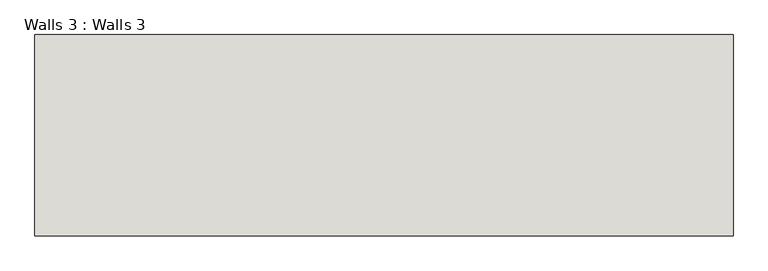
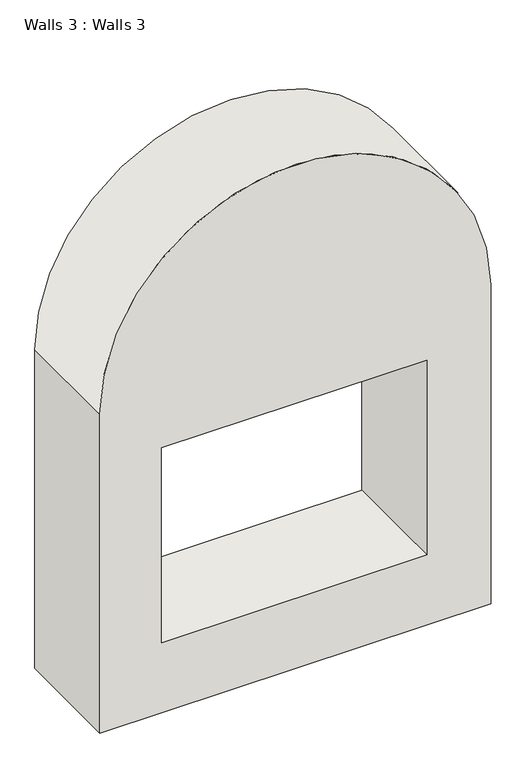
"""IFC4 building model written with IfcOpenShell, lengths in millimetres: wall geometry, Walls 3 : Walls 3."""

from ifc_helpers import new_model, si_unit, point, frame, frame_2d, origin, place, context, project, spatial, polyline, circle_curve, trimmed, segment, composite_curve, outline, extrude, source, transform, mapped, element, save


def walls_3_walls_3_3787e265(model_context):
    return source(origin(), model_context, "Body", "SweptSolid", [
        extrude(outline(composite_curve([segment(polyline([(3048.0, 7266.7445455), (3048.0, 9716.964129), (5159.6397851, 9716.964129)]), True, "CONTINUOUS"), segment(trimmed(circle_curve(frame_2d((5159.6397851, 8491.8543372)), 1225.1097918), [point((5159.6397851, 9716.964129))], [point((5159.6397851, 7266.7445455))], False, "CARTESIAN"), True, "CONTINUOUS"), segment(polyline([(5159.6397851, 7266.7445455), (3048.0, 7266.7445455)]), True, "CONTINUOUS")], self_intersect=False), holes=[polyline([(3511.4578847, 7652.9761575), (4800.5078847, 7652.9761575), (4800.5078847, 9316.6761575), (3511.4578847, 9316.6761575), (3511.4578847, 7652.9761575)])]), frame((0.0, -3844.6250111, 0.0), z_axis=(0.0, 1.0, 0.0), x_axis=(0.0, 0.0, 1.0)), (0.0, 0.0, 1.0), 705.8739186),
    ])


if __name__ == "__main__":
    model = new_model("IFC4")
    model_context = context("Model", 3, world=origin())
    ifc_project = project(units=[si_unit("LENGTHUNIT", "METRE", prefix="MILLI")], contexts=[model_context])
    site = spatial("IfcSite", under=ifc_project)
    building = spatial("IfcBuilding", under=site)
    placement = place(None, origin())
    walls_3_walls_3_shape = walls_3_walls_3_3787e265(model_context)
    element("IfcWall", 1, ObjectType="Walls 3 : Walls 3", at=placement, inside=building, context=model_context, shape_type="MappedRepresentation", body=[
        mapped(walls_3_walls_3_shape, transform((0.0, 0.0, 0.0), x_axis=(1.0, 0.0, 0.0), y_axis=(0.0, 1.0, 0.0), z_axis=(0.0, 0.0, 1.0))),
    ])
    save(model, "model.ifc")

# Revit data of these elements
# Element 1 (IfcWall, "Walls 3 : Walls 3")
#   Materials on its faces: "Default Wall"
# Materials
#   "Default Wall": colour RGB 80 80 80, transparency 0
